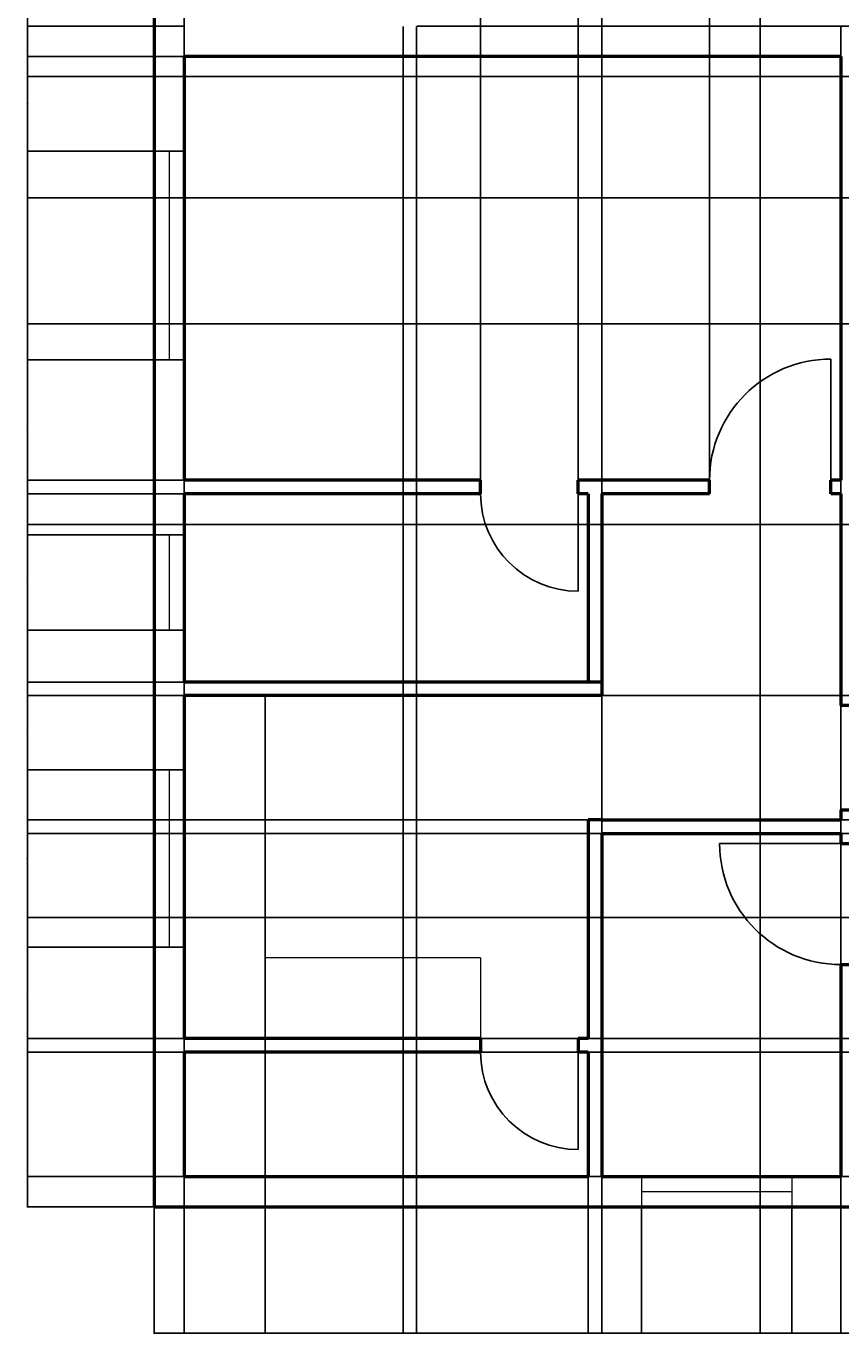
# Model space of a CAD drawing. Units: inches. Extents: x 2479 to 3284, y 2154 to 2936.
# Tile 1 of 8: x 2479 to 2721, y 2154 to 2543. Entities that reach past the tile are written whole.
import ezdxf

# ---------------------------------------------------------------- set-up
doc = ezdxf.new("R2010")
doc.units = ezdxf.units.IN
for name, color, linetype, lineweight in [('A-ANNO-DIMS', 2, 'Continuous', 18), ('A-DOOR', 3, 'Continuous', 25), ('A-FLOR-CASE', 8, 'Continuous', 18), ('A-GLAZ', 4, 'Continuous', 18), ('A-WALL', 7, 'Continuous', 50)]:
    doc.layers.add(name, color=color, linetype=linetype, lineweight=lineweight)
doc.styles.get("Standard").update_dxf_attribs({"font": 'arial.ttf'})
doc.dimstyles.get("Standard").update_dxf_attribs({"dimtxt": 0.18, "dimasz": 0.18, "dimexe": 0.18, "dimexo": 0.0625, "dimgap": 0.09, "dimtad": 0, "dimtih": 1, "dimtoh": 1, "dimdec": 4, "dimzin": 0, "dimdsep": 46, "dimtxsty": 'Standard', "dimcen": 0.09, "dimadec": 0, "dimazin": 0, "dimtfac": 1, "dimtdec": 4, "dimtofl": 0, "dimtmove": 0, "dimatfit": 3, "dimfxl": 1, "dimtolj": 1, "dimtzin": 0, "dimarcsym": 0})

# ---------------------------------------------------------------- blocks, each defined once
blk = doc.blocks.new('DOOR-SWING-29IN')
blk.add_line((29, 0), (0, 0))
blk.add_arc((29, 0), 29, 90, 180)
blk = doc.blocks.new('DOOR-SWING-36IN')
blk.add_line((36, 0), (0, 0))
blk.add_arc((36, 0), 36, 90, 180)
blk = doc.blocks.new('*D7')
at = {"layer": 'A-ANNO-DIMS', "color": 0, "lineweight": -2, "transparency": 16777216}
for p, q in [((2517.21, 2191.68), (2517.21, 2153.96)), ((3246.21, 2191.68), (3246.21, 2153.96)), ((2517.39, 2154.14), (2881.42, 2154.14)), ((3246.03, 2154.14), (2882, 2154.14))]:
    blk.add_line(p, q, dxfattribs=at)
at = {"layer": 'A-ANNO-DIMS', "color": 0, "transparency": 16777216}
for points in [[(2517.39, 2154.17), (2517.39, 2154.11), (2517.21, 2154.14)], [(3246.03, 2154.17), (3246.03, 2154.11), (3246.21, 2154.14)]]:
    blk.add_solid(points, dxfattribs=at)
at = {"layer": 'Defpoints', "color": 0, "transparency": 16777216}
for p in [(2517.21, 2191.74), (3246.21, 2191.74), (3246.21, 2154.14)]:
    blk.add_point(p, dxfattribs=at)
at = {"layer": 'A-ANNO-DIMS', "color": 0, "transparency": 16777216, "insert": (2881.71, 2154.14), "char_height": 0.18, "attachment_point": 5}
blk.add_mtext('\\A1;729', dxfattribs=at)
blk = doc.blocks.new('*D8')
at = {"layer": 'A-ANNO-DIMS', "color": 0, "lineweight": -2, "transparency": 16777216}
for p, q in [((2517.15, 2897.74), (2479.43, 2897.74)), ((2479.61, 2897.56), (2479.61, 2544.92)), ((2479.61, 2191.92), (2479.61, 2544.56)), ((2517.15, 2191.74), (2479.43, 2191.74))]:
    blk.add_line(p, q, dxfattribs=at)
at = {"layer": 'A-ANNO-DIMS', "color": 0, "transparency": 16777216}
for points in [[(2479.58, 2897.56), (2479.64, 2897.56), (2479.61, 2897.74)], [(2479.58, 2191.92), (2479.64, 2191.92), (2479.61, 2191.74)]]:
    blk.add_solid(points, dxfattribs=at)
at = {"layer": 'Defpoints', "color": 0, "transparency": 16777216}
for p in [(2479.61, 2897.74), (2517.21, 2897.74), (2517.21, 2191.74)]:
    blk.add_point(p, dxfattribs=at)
at = {"layer": 'A-ANNO-DIMS', "color": 0, "transparency": 16777216, "insert": (2479.61, 2544.74), "char_height": 0.18, "attachment_point": 5}
blk.add_mtext('\\A1;706', dxfattribs=at)
blk = doc.blocks.new('*D24')
at = {"layer": 'A-ANNO-DIMS', "color": 0, "lineweight": -2, "transparency": 16777216}
for p, q in [((2845.15, 2394.59), (2479.43, 2394.59)), ((2479.61, 2394.41), (2479.61, 2336.35)), ((2479.61, 2277.92), (2479.61, 2335.98)), ((2845.15, 2277.74), (2479.43, 2277.74))]:
    blk.add_line(p, q, dxfattribs=at)
at = {"layer": 'A-ANNO-DIMS', "color": 0, "transparency": 16777216}
for points in [[(2479.58, 2394.41), (2479.64, 2394.41), (2479.61, 2394.59)], [(2479.58, 2277.92), (2479.64, 2277.92), (2479.61, 2277.74)]]:
    blk.add_solid(points, dxfattribs=at)
at = {"layer": 'Defpoints', "color": 0, "transparency": 16777216}
for p in [(2479.61, 2394.59), (2845.21, 2394.59), (2845.21, 2277.74)]:
    blk.add_point(p, dxfattribs=at)
at = {"layer": 'A-ANNO-DIMS', "color": 0, "transparency": 16777216, "insert": (2479.61, 2336.17), "char_height": 0.18, "attachment_point": 5}
blk.add_mtext('\\A1;116.85', dxfattribs=at)
blk = doc.blocks.new('*D25')
at = {"layer": 'A-ANNO-DIMS', "color": 0, "lineweight": -2, "transparency": 16777216}
for p, q in [((2845.15, 2454.21), (2479.43, 2454.21)), ((2479.61, 2454.03), (2479.61, 2424.58)), ((2479.61, 2394.77), (2479.61, 2424.22)), ((2845.15, 2394.59), (2479.43, 2394.59))]:
    blk.add_line(p, q, dxfattribs=at)
at = {"layer": 'A-ANNO-DIMS', "color": 0, "transparency": 16777216}
for points in [[(2479.58, 2454.03), (2479.64, 2454.03), (2479.61, 2454.21)], [(2479.58, 2394.77), (2479.64, 2394.77), (2479.61, 2394.59)]]:
    blk.add_solid(points, dxfattribs=at)
at = {"layer": 'Defpoints', "color": 0, "transparency": 16777216}
for p in [(2479.61, 2454.21), (2845.21, 2454.21), (2845.21, 2394.59)]:
    blk.add_point(p, dxfattribs=at)
at = {"layer": 'A-ANNO-DIMS', "color": 0, "transparency": 16777216, "insert": (2479.61, 2424.4), "char_height": 0.18, "attachment_point": 5}
blk.add_mtext('\\A1;59.61', dxfattribs=at)
blk = doc.blocks.new('*D26')
at = {"layer": 'A-ANNO-DIMS', "color": 0, "lineweight": -2, "transparency": 16777216}
for p, q in [((2845.15, 2491.74), (2479.43, 2491.74)), ((2479.61, 2491.56), (2479.61, 2473.15)), ((2479.61, 2454.39), (2479.61, 2472.79)), ((2845.15, 2454.21), (2479.43, 2454.21))]:
    blk.add_line(p, q, dxfattribs=at)
at = {"layer": 'A-ANNO-DIMS', "color": 0, "transparency": 16777216}
for points in [[(2479.58, 2491.56), (2479.64, 2491.56), (2479.61, 2491.74)], [(2479.58, 2454.39), (2479.64, 2454.39), (2479.61, 2454.21)]]:
    blk.add_solid(points, dxfattribs=at)
at = {"layer": 'Defpoints', "color": 0, "transparency": 16777216}
for p in [(2479.61, 2491.74), (2845.21, 2491.74), (2845.21, 2454.21)]:
    blk.add_point(p, dxfattribs=at)
at = {"layer": 'A-ANNO-DIMS', "color": 0, "transparency": 16777216, "insert": (2479.61, 2472.97), "char_height": 0.18, "attachment_point": 5}
blk.add_mtext('\\A1;37.534', dxfattribs=at)
blk = doc.blocks.new('*D27')
at = {"layer": 'A-ANNO-DIMS', "color": 0, "lineweight": -2, "transparency": 16777216}
for p, q in [((2845.15, 2545.74), (2479.43, 2545.74)), ((2479.61, 2545.56), (2479.61, 2536.92)), ((2479.61, 2527.92), (2479.61, 2536.56)), ((2845.15, 2527.74), (2479.43, 2527.74))]:
    blk.add_line(p, q, dxfattribs=at)
at = {"layer": 'A-ANNO-DIMS', "color": 0, "transparency": 16777216}
for points in [[(2479.58, 2545.56), (2479.64, 2545.56), (2479.61, 2545.74)], [(2479.58, 2527.92), (2479.64, 2527.92), (2479.61, 2527.74)]]:
    blk.add_solid(points, dxfattribs=at)
at = {"layer": 'Defpoints', "color": 0, "transparency": 16777216}
for p in [(2479.61, 2545.74), (2845.21, 2545.74), (2845.21, 2527.74)]:
    blk.add_point(p, dxfattribs=at)
at = {"layer": 'A-ANNO-DIMS', "color": 0, "transparency": 16777216, "insert": (2479.61, 2536.74), "char_height": 0.18, "attachment_point": 5}
blk.add_mtext('\\A1;18', dxfattribs=at)
blk = doc.blocks.new('*D48')
at = {"layer": 'A-ANNO-DIMS', "color": 0, "lineweight": -2, "transparency": 16777216}
for p, q in [((2526.21, 2542.68), (2526.21, 2153.96)), ((2591.21, 2542.68), (2591.21, 2153.96)), ((2526.39, 2154.14), (2558.49, 2154.14)), ((2591.03, 2154.14), (2558.93, 2154.14))]:
    blk.add_line(p, q, dxfattribs=at)
at = {"layer": 'A-ANNO-DIMS', "color": 0, "transparency": 16777216}
for points in [[(2526.39, 2154.17), (2526.39, 2154.11), (2526.21, 2154.14)], [(2591.03, 2154.17), (2591.03, 2154.11), (2591.21, 2154.14)]]:
    blk.add_solid(points, dxfattribs=at)
at = {"layer": 'Defpoints', "color": 0, "transparency": 16777216}
for p in [(2526.21, 2542.74), (2591.21, 2542.74), (2591.21, 2154.14)]:
    blk.add_point(p, dxfattribs=at)
at = {"layer": 'A-ANNO-DIMS', "color": 0, "transparency": 16777216, "insert": (2558.71, 2154.14), "char_height": 0.18, "attachment_point": 5}
blk.add_mtext('\\A1;65', dxfattribs=at)
blk = doc.blocks.new('*D49')
at = {"layer": 'A-ANNO-DIMS', "color": 0, "lineweight": -2, "transparency": 16777216}
for p, q in [((2595.21, 2542.68), (2595.21, 2153.96)), ((2721.21, 2542.68), (2721.21, 2153.96)), ((2595.39, 2154.14), (2657.93, 2154.14)), ((2721.03, 2154.14), (2658.49, 2154.14))]:
    blk.add_line(p, q, dxfattribs=at)
at = {"layer": 'A-ANNO-DIMS', "color": 0, "transparency": 16777216}
for points in [[(2595.39, 2154.17), (2595.39, 2154.11), (2595.21, 2154.14)], [(2721.03, 2154.17), (2721.03, 2154.11), (2721.21, 2154.14)]]:
    blk.add_solid(points, dxfattribs=at)
at = {"layer": 'Defpoints', "color": 0, "transparency": 16777216}
for p in [(2595.21, 2542.74), (2721.21, 2542.74), (2721.21, 2154.14)]:
    blk.add_point(p, dxfattribs=at)
at = {"layer": 'A-ANNO-DIMS', "color": 0, "transparency": 16777216, "insert": (2658.21, 2154.14), "char_height": 0.18, "attachment_point": 5}
blk.add_mtext('\\A1;126', dxfattribs=at)
blk = doc.blocks.new('*D51')
at = {"layer": 'A-ANNO-DIMS', "color": 0, "lineweight": -2, "transparency": 16777216}
for p, q in [((2526.15, 2638.74), (2479.43, 2638.74)), ((2479.61, 2638.56), (2479.61, 2590.92)), ((2479.61, 2542.92), (2479.61, 2590.56)), ((2526.15, 2542.74), (2479.43, 2542.74))]:
    blk.add_line(p, q, dxfattribs=at)
at = {"layer": 'A-ANNO-DIMS', "color": 0, "transparency": 16777216}
for points in [[(2479.58, 2638.56), (2479.64, 2638.56), (2479.61, 2638.74)], [(2479.58, 2542.92), (2479.64, 2542.92), (2479.61, 2542.74)]]:
    blk.add_solid(points, dxfattribs=at)
at = {"layer": 'Defpoints', "color": 0, "transparency": 16777216}
for p in [(2479.61, 2638.74), (2526.21, 2638.74), (2526.21, 2542.74)]:
    blk.add_point(p, dxfattribs=at)
at = {"layer": 'A-ANNO-DIMS', "color": 0, "transparency": 16777216, "insert": (2479.61, 2590.74), "char_height": 0.18, "attachment_point": 5}
blk.add_mtext('\\A1;96', dxfattribs=at)
blk = doc.blocks.new('*D61')
at = {"layer": 'A-ANNO-DIMS', "color": 0, "lineweight": -2, "transparency": 16777216}
for p, q in [((2595.27, 2566.74), (3283.99, 2566.74)), ((3283.81, 2566.56), (3283.81, 2554.92)), ((3283.81, 2542.92), (3283.81, 2554.56)), ((2595.27, 2542.74), (3283.99, 2542.74))]:
    blk.add_line(p, q, dxfattribs=at)
at = {"layer": 'A-ANNO-DIMS', "color": 0, "transparency": 16777216}
for points in [[(3283.78, 2566.56), (3283.84, 2566.56), (3283.81, 2566.74)], [(3283.78, 2542.92), (3283.84, 2542.92), (3283.81, 2542.74)]]:
    blk.add_solid(points, dxfattribs=at)
at = {"layer": 'Defpoints', "color": 0, "transparency": 16777216}
for p in [(2595.21, 2566.74), (3283.81, 2566.74), (2595.21, 2542.74)]:
    blk.add_point(p, dxfattribs=at)
at = {"layer": 'A-ANNO-DIMS', "color": 0, "transparency": 16777216, "insert": (3283.81, 2554.74), "char_height": 0.18, "attachment_point": 5}
blk.add_mtext('\\A1;24', dxfattribs=at)
blk = doc.blocks.new('*D63')
at = {"layer": 'A-ANNO-DIMS', "color": 0, "lineweight": -2, "transparency": 16777216}
for p, q in [((2650.21, 2642.68), (2650.21, 2153.96)), ((2697.21, 2642.68), (2697.21, 2153.96)), ((2650.39, 2154.14), (2673.49, 2154.14)), ((2697.03, 2154.14), (2673.93, 2154.14))]:
    blk.add_line(p, q, dxfattribs=at)
at = {"layer": 'A-ANNO-DIMS', "color": 0, "transparency": 16777216}
for points in [[(2650.39, 2154.17), (2650.39, 2154.11), (2650.21, 2154.14)], [(2697.03, 2154.17), (2697.03, 2154.11), (2697.21, 2154.14)]]:
    blk.add_solid(points, dxfattribs=at)
at = {"layer": 'Defpoints', "color": 0, "transparency": 16777216}
for p in [(2650.21, 2642.74), (2697.21, 2642.74), (2697.21, 2154.14)]:
    blk.add_point(p, dxfattribs=at)
at = {"layer": 'A-ANNO-DIMS', "color": 0, "transparency": 16777216, "insert": (2673.71, 2154.14), "char_height": 0.18, "attachment_point": 5}
blk.add_mtext('\\A1;47', dxfattribs=at)
blk = doc.blocks.new('*D90')
at = {"layer": 'A-ANNO-DIMS', "color": 0, "lineweight": -2, "transparency": 16777216}
for p, q in [((2526.21, 2200.68), (2526.21, 2153.96)), ((2646.21, 2200.68), (2646.21, 2153.96)), ((2526.39, 2154.14), (2585.93, 2154.14)), ((2646.03, 2154.14), (2586.49, 2154.14))]:
    blk.add_line(p, q, dxfattribs=at)
at = {"layer": 'A-ANNO-DIMS', "color": 0, "transparency": 16777216}
for points in [[(2526.39, 2154.17), (2526.39, 2154.11), (2526.21, 2154.14)], [(2646.03, 2154.17), (2646.03, 2154.11), (2646.21, 2154.14)]]:
    blk.add_solid(points, dxfattribs=at)
at = {"layer": 'Defpoints', "color": 0, "transparency": 16777216}
for p in [(2526.21, 2200.74), (2646.21, 2200.74), (2646.21, 2154.14)]:
    blk.add_point(p, dxfattribs=at)
at = {"layer": 'A-ANNO-DIMS', "color": 0, "transparency": 16777216, "insert": (2586.21, 2154.14), "char_height": 0.18, "attachment_point": 5}
blk.add_mtext('\\A1;120', dxfattribs=at)
blk = doc.blocks.new('*D91')
at = {"layer": 'A-ANNO-DIMS', "color": 0, "lineweight": -2, "transparency": 16777216}
for p, q in [((2650.21, 2200.68), (2650.21, 2153.96)), ((2661.98, 2191.68), (2661.98, 2153.96)), ((2650.39, 2154.14), (2655.71, 2154.14)), ((2661.8, 2154.14), (2656.48, 2154.14))]:
    blk.add_line(p, q, dxfattribs=at)
at = {"layer": 'A-ANNO-DIMS', "color": 0, "transparency": 16777216}
for points in [[(2650.39, 2154.17), (2650.39, 2154.11), (2650.21, 2154.14)], [(2661.8, 2154.17), (2661.8, 2154.11), (2661.98, 2154.14)]]:
    blk.add_solid(points, dxfattribs=at)
at = {"layer": 'Defpoints', "color": 0, "transparency": 16777216}
for p in [(2650.21, 2200.74), (2661.98, 2191.74), (2661.98, 2154.14)]:
    blk.add_point(p, dxfattribs=at)
at = {"layer": 'A-ANNO-DIMS', "color": 0, "transparency": 16777216, "insert": (2656.09, 2154.14), "char_height": 0.18, "attachment_point": 5}
blk.add_mtext('\\A1;11.77', dxfattribs=at)
blk = doc.blocks.new('*D92')
at = {"layer": 'A-ANNO-DIMS', "color": 0, "lineweight": -2, "transparency": 16777216}
for p, q in [((2661.98, 2191.68), (2661.98, 2153.96)), ((2706.69, 2191.68), (2706.69, 2153.96)), ((2662.16, 2154.14), (2683.96, 2154.14)), ((2706.51, 2154.14), (2684.71, 2154.14))]:
    blk.add_line(p, q, dxfattribs=at)
at = {"layer": 'A-ANNO-DIMS', "color": 0, "transparency": 16777216}
for points in [[(2662.16, 2154.17), (2662.16, 2154.11), (2661.98, 2154.14)], [(2706.51, 2154.17), (2706.51, 2154.11), (2706.69, 2154.14)]]:
    blk.add_solid(points, dxfattribs=at)
at = {"layer": 'Defpoints', "color": 0, "transparency": 16777216}
for p in [(2661.98, 2191.74), (2706.69, 2191.74), (2706.69, 2154.14)]:
    blk.add_point(p, dxfattribs=at)
at = {"layer": 'A-ANNO-DIMS', "color": 0, "transparency": 16777216, "insert": (2684.33, 2154.14), "char_height": 0.18, "attachment_point": 5}
blk.add_mtext('\\A1;44.71', dxfattribs=at)
blk = doc.blocks.new('*D93')
at = {"layer": 'A-ANNO-DIMS', "color": 0, "lineweight": -2, "transparency": 16777216}
for p, q in [((2721.21, 2200.68), (2721.21, 2153.96)), ((2706.69, 2191.68), (2706.69, 2153.96)), ((2706.87, 2154.14), (2713.49, 2154.14)), ((2721.03, 2154.14), (2714.41, 2154.14))]:
    blk.add_line(p, q, dxfattribs=at)
at = {"layer": 'A-ANNO-DIMS', "color": 0, "transparency": 16777216}
for points in [[(2706.87, 2154.17), (2706.87, 2154.11), (2706.69, 2154.14)], [(2721.03, 2154.17), (2721.03, 2154.11), (2721.21, 2154.14)]]:
    blk.add_solid(points, dxfattribs=at)
at = {"layer": 'Defpoints', "color": 0, "transparency": 16777216}
for p in [(2721.21, 2200.74), (2706.69, 2191.74), (2721.21, 2154.14)]:
    blk.add_point(p, dxfattribs=at)
at = {"layer": 'A-ANNO-DIMS', "color": 0, "transparency": 16777216, "insert": (2713.95, 2154.14), "char_height": 0.18, "attachment_point": 5}
blk.add_mtext('\\A1;14.518', dxfattribs=at)
blk = doc.blocks.new('*D96')
at = {"layer": 'A-ANNO-DIMS', "color": 0, "lineweight": -2, "transparency": 16777216}
for p, q in [((2526.15, 2237.74), (2479.43, 2237.74)), ((2479.61, 2237.56), (2479.61, 2219.42)), ((2479.61, 2200.92), (2479.61, 2219.06)), ((2526.15, 2200.74), (2479.43, 2200.74))]:
    blk.add_line(p, q, dxfattribs=at)
at = {"layer": 'A-ANNO-DIMS', "color": 0, "transparency": 16777216}
for points in [[(2479.58, 2237.56), (2479.64, 2237.56), (2479.61, 2237.74)], [(2479.58, 2200.92), (2479.64, 2200.92), (2479.61, 2200.74)]]:
    blk.add_solid(points, dxfattribs=at)
at = {"layer": 'Defpoints', "color": 0, "transparency": 16777216}
for p in [(2479.61, 2237.74), (2526.21, 2237.74), (2526.21, 2200.74)]:
    blk.add_point(p, dxfattribs=at)
at = {"layer": 'A-ANNO-DIMS', "color": 0, "transparency": 16777216, "insert": (2479.61, 2219.24), "char_height": 0.18, "attachment_point": 5}
blk.add_mtext('\\A1;37', dxfattribs=at)
blk = doc.blocks.new('*D97')
at = {"layer": 'A-ANNO-DIMS', "color": 0, "lineweight": -2, "transparency": 16777216}
for p, q in [((2526.15, 2268.88), (2479.43, 2268.88)), ((2479.61, 2268.7), (2479.61, 2255.49)), ((2479.61, 2241.92), (2479.61, 2255.13)), ((2526.15, 2241.74), (2479.43, 2241.74))]:
    blk.add_line(p, q, dxfattribs=at)
at = {"layer": 'A-ANNO-DIMS', "color": 0, "transparency": 16777216}
for points in [[(2479.58, 2268.7), (2479.64, 2268.7), (2479.61, 2268.88)], [(2479.58, 2241.92), (2479.64, 2241.92), (2479.61, 2241.74)]]:
    blk.add_solid(points, dxfattribs=at)
at = {"layer": 'Defpoints', "color": 0, "transparency": 16777216}
for p in [(2479.61, 2268.88), (2526.21, 2268.88), (2526.21, 2241.74)]:
    blk.add_point(p, dxfattribs=at)
at = {"layer": 'A-ANNO-DIMS', "color": 0, "transparency": 16777216, "insert": (2479.61, 2255.31), "char_height": 0.18, "attachment_point": 5}
blk.add_mtext('\\A1;27.14', dxfattribs=at)
blk = doc.blocks.new('*D98')
at = {"layer": 'A-ANNO-DIMS', "color": 0, "lineweight": -2, "transparency": 16777216}
for p, q in [((2526.15, 2321.65), (2479.43, 2321.65)), ((2479.61, 2321.47), (2479.61, 2295.44)), ((2479.61, 2269.06), (2479.61, 2295.08)), ((2526.15, 2268.88), (2479.43, 2268.88))]:
    blk.add_line(p, q, dxfattribs=at)
at = {"layer": 'A-ANNO-DIMS', "color": 0, "transparency": 16777216}
for points in [[(2479.58, 2321.47), (2479.64, 2321.47), (2479.61, 2321.65)], [(2479.58, 2269.06), (2479.64, 2269.06), (2479.61, 2268.88)]]:
    blk.add_solid(points, dxfattribs=at)
at = {"layer": 'Defpoints', "color": 0, "transparency": 16777216}
for p in [(2479.61, 2321.65), (2526.21, 2321.65), (2526.21, 2268.88)]:
    blk.add_point(p, dxfattribs=at)
at = {"layer": 'A-ANNO-DIMS', "color": 0, "transparency": 16777216, "insert": (2479.61, 2295.26), "char_height": 0.18, "attachment_point": 5}
blk.add_mtext('\\A1;52.76', dxfattribs=at)
blk = doc.blocks.new('*D99')
at = {"layer": 'A-ANNO-DIMS', "color": 0, "lineweight": -2, "transparency": 16777216}
for p, q in [((2526.15, 2343.74), (2479.43, 2343.74)), ((2479.61, 2343.56), (2479.61, 2332.87)), ((2479.61, 2321.83), (2479.61, 2332.51)), ((2526.15, 2321.65), (2479.43, 2321.65))]:
    blk.add_line(p, q, dxfattribs=at)
at = {"layer": 'A-ANNO-DIMS', "color": 0, "transparency": 16777216}
for points in [[(2479.58, 2343.56), (2479.64, 2343.56), (2479.61, 2343.74)], [(2479.58, 2321.83), (2479.64, 2321.83), (2479.61, 2321.65)]]:
    blk.add_solid(points, dxfattribs=at)
at = {"layer": 'Defpoints', "color": 0, "transparency": 16777216}
for p in [(2479.61, 2343.74), (2526.21, 2343.74), (2526.21, 2321.65)]:
    blk.add_point(p, dxfattribs=at)
at = {"layer": 'A-ANNO-DIMS', "color": 0, "transparency": 16777216, "insert": (2479.61, 2332.69), "char_height": 0.18, "attachment_point": 5}
blk.add_mtext('\\A1;22.095', dxfattribs=at)
blk = doc.blocks.new('*D100')
at = {"layer": 'A-ANNO-DIMS', "color": 0, "lineweight": -2, "transparency": 16777216}
for p, q in [((2526.15, 2363.18), (2479.43, 2363.18)), ((2479.61, 2363), (2479.61, 2355.64)), ((2479.61, 2347.92), (2479.61, 2355.28)), ((2526.15, 2347.74), (2479.43, 2347.74))]:
    blk.add_line(p, q, dxfattribs=at)
at = {"layer": 'A-ANNO-DIMS', "color": 0, "transparency": 16777216}
for points in [[(2479.58, 2363), (2479.64, 2363), (2479.61, 2363.18)], [(2479.58, 2347.92), (2479.64, 2347.92), (2479.61, 2347.74)]]:
    blk.add_solid(points, dxfattribs=at)
at = {"layer": 'Defpoints', "color": 0, "transparency": 16777216}
for p in [(2479.61, 2363.18), (2526.21, 2363.18), (2526.21, 2347.74)]:
    blk.add_point(p, dxfattribs=at)
at = {"layer": 'A-ANNO-DIMS', "color": 0, "transparency": 16777216, "insert": (2479.61, 2355.46), "char_height": 0.18, "attachment_point": 5}
blk.add_mtext('\\A1;15.44', dxfattribs=at)
blk = doc.blocks.new('*D101')
at = {"layer": 'A-ANNO-DIMS', "color": 0, "lineweight": -2, "transparency": 16777216}
for p, q in [((2526.15, 2391.55), (2479.43, 2391.55)), ((2479.61, 2391.37), (2479.61, 2377.55)), ((2479.61, 2363.36), (2479.61, 2377.18)), ((2526.15, 2363.18), (2479.43, 2363.18))]:
    blk.add_line(p, q, dxfattribs=at)
at = {"layer": 'A-ANNO-DIMS', "color": 0, "transparency": 16777216}
for points in [[(2479.58, 2391.37), (2479.64, 2391.37), (2479.61, 2391.55)], [(2479.58, 2363.36), (2479.64, 2363.36), (2479.61, 2363.18)]]:
    blk.add_solid(points, dxfattribs=at)
at = {"layer": 'Defpoints', "color": 0, "transparency": 16777216}
for p in [(2479.61, 2391.55), (2526.21, 2391.55), (2526.21, 2363.18)]:
    blk.add_point(p, dxfattribs=at)
at = {"layer": 'A-ANNO-DIMS', "color": 0, "transparency": 16777216, "insert": (2479.61, 2377.37), "char_height": 0.18, "attachment_point": 5}
blk.add_mtext('\\A1;28.376', dxfattribs=at)
blk = doc.blocks.new('*D102')
at = {"layer": 'A-ANNO-DIMS', "color": 0, "lineweight": -2, "transparency": 16777216}
for p, q in [((2526.15, 2403.74), (2479.43, 2403.74)), ((2479.61, 2403.56), (2479.61, 2397.83)), ((2479.61, 2391.73), (2479.61, 2397.47)), ((2526.15, 2391.55), (2479.43, 2391.55))]:
    blk.add_line(p, q, dxfattribs=at)
at = {"layer": 'A-ANNO-DIMS', "color": 0, "transparency": 16777216}
for points in [[(2479.58, 2403.56), (2479.64, 2403.56), (2479.61, 2403.74)], [(2479.58, 2391.73), (2479.64, 2391.73), (2479.61, 2391.55)]]:
    blk.add_solid(points, dxfattribs=at)
at = {"layer": 'Defpoints', "color": 0, "transparency": 16777216}
for p in [(2479.61, 2403.74), (2526.21, 2403.74), (2526.21, 2391.55)]:
    blk.add_point(p, dxfattribs=at)
at = {"layer": 'A-ANNO-DIMS', "color": 0, "transparency": 16777216, "insert": (2479.61, 2397.65), "char_height": 0.18, "attachment_point": 5}
blk.add_mtext('\\A1;12.185', dxfattribs=at)
blk = doc.blocks.new('*D103')
at = {"layer": 'A-ANNO-DIMS', "color": 0, "lineweight": -2, "transparency": 16777216}
for p, q in [((2526.15, 2443.49), (2479.43, 2443.49)), ((2479.61, 2443.31), (2479.61, 2425.8)), ((2479.61, 2407.92), (2479.61, 2425.43)), ((2526.15, 2407.74), (2479.43, 2407.74))]:
    blk.add_line(p, q, dxfattribs=at)
at = {"layer": 'A-ANNO-DIMS', "color": 0, "transparency": 16777216}
for points in [[(2479.58, 2443.31), (2479.64, 2443.31), (2479.61, 2443.49)], [(2479.58, 2407.92), (2479.64, 2407.92), (2479.61, 2407.74)]]:
    blk.add_solid(points, dxfattribs=at)
at = {"layer": 'Defpoints', "color": 0, "transparency": 16777216}
for p in [(2479.61, 2443.49), (2526.21, 2443.49), (2526.21, 2407.74)]:
    blk.add_point(p, dxfattribs=at)
at = {"layer": 'A-ANNO-DIMS', "color": 0, "transparency": 16777216, "insert": (2479.61, 2425.61), "char_height": 0.18, "attachment_point": 5}
blk.add_mtext('\\A1;35.75', dxfattribs=at)
blk = doc.blocks.new('*D104')
at = {"layer": 'A-ANNO-DIMS', "color": 0, "lineweight": -2, "transparency": 16777216}
for p, q in [((2526.15, 2505.53), (2479.43, 2505.53)), ((2479.61, 2505.35), (2479.61, 2474.69)), ((2479.61, 2443.67), (2479.61, 2474.33)), ((2526.15, 2443.49), (2479.43, 2443.49))]:
    blk.add_line(p, q, dxfattribs=at)
at = {"layer": 'A-ANNO-DIMS', "color": 0, "transparency": 16777216}
for points in [[(2479.58, 2505.35), (2479.64, 2505.35), (2479.61, 2505.53)], [(2479.58, 2443.67), (2479.64, 2443.67), (2479.61, 2443.49)]]:
    blk.add_solid(points, dxfattribs=at)
at = {"layer": 'Defpoints', "color": 0, "transparency": 16777216}
for p in [(2479.61, 2505.53), (2526.21, 2505.53), (2526.21, 2443.49)]:
    blk.add_point(p, dxfattribs=at)
at = {"layer": 'A-ANNO-DIMS', "color": 0, "transparency": 16777216, "insert": (2479.61, 2474.51), "char_height": 0.18, "attachment_point": 5}
blk.add_mtext('\\A1;62.05', dxfattribs=at)
blk = doc.blocks.new('*D105')
at = {"layer": 'A-ANNO-DIMS', "color": 0, "lineweight": -2, "transparency": 16777216}
for p, q in [((2526.15, 2533.74), (2479.43, 2533.74)), ((2479.61, 2533.56), (2479.61, 2519.82)), ((2479.61, 2505.71), (2479.61, 2519.46)), ((2526.15, 2505.53), (2479.43, 2505.53))]:
    blk.add_line(p, q, dxfattribs=at)
at = {"layer": 'A-ANNO-DIMS', "color": 0, "transparency": 16777216}
for points in [[(2479.58, 2533.56), (2479.64, 2533.56), (2479.61, 2533.74)], [(2479.58, 2505.71), (2479.64, 2505.71), (2479.61, 2505.53)]]:
    blk.add_solid(points, dxfattribs=at)
at = {"layer": 'Defpoints', "color": 0, "transparency": 16777216}
for p in [(2479.61, 2533.74), (2526.21, 2533.74), (2526.21, 2505.53)]:
    blk.add_point(p, dxfattribs=at)
at = {"layer": 'A-ANNO-DIMS', "color": 0, "transparency": 16777216, "insert": (2479.61, 2519.64), "char_height": 0.18, "attachment_point": 5}
blk.add_mtext('\\A1;28.205', dxfattribs=at)
blk = doc.blocks.new('*D109')
at = {"layer": 'A-ANNO-DIMS', "color": 0, "lineweight": -2, "transparency": 16777216}
for p, q in [((2526.21, 2407.8), (2526.21, 2935.52)), ((2526.39, 2935.34), (2569.99, 2935.34)), ((2614.03, 2935.34), (2570.43, 2935.34)), ((2614.21, 2407.8), (2614.21, 2935.52))]:
    blk.add_line(p, q, dxfattribs=at)
at = {"layer": 'A-ANNO-DIMS', "color": 0, "transparency": 16777216}
for points in [[(2526.39, 2935.37), (2526.39, 2935.31), (2526.21, 2935.34)], [(2614.03, 2935.37), (2614.03, 2935.31), (2614.21, 2935.34)]]:
    blk.add_solid(points, dxfattribs=at)
at = {"layer": 'Defpoints', "color": 0, "transparency": 16777216}
for p in [(2614.21, 2935.34), (2526.21, 2407.74), (2614.21, 2407.74)]:
    blk.add_point(p, dxfattribs=at)
at = {"layer": 'A-ANNO-DIMS', "color": 0, "transparency": 16777216, "insert": (2570.21, 2935.34), "char_height": 0.18, "attachment_point": 5}
blk.add_mtext('\\A1;88', dxfattribs=at)
blk = doc.blocks.new('*D110')
at = {"layer": 'A-ANNO-DIMS', "color": 0, "lineweight": -2, "transparency": 16777216}
for p, q in [((2643.21, 2407.8), (2643.21, 2935.52)), ((2643.39, 2935.34), (2662.49, 2935.34)), ((2682.03, 2935.34), (2662.93, 2935.34)), ((2682.21, 2407.8), (2682.21, 2935.52))]:
    blk.add_line(p, q, dxfattribs=at)
at = {"layer": 'A-ANNO-DIMS', "color": 0, "transparency": 16777216}
for points in [[(2643.39, 2935.37), (2643.39, 2935.31), (2643.21, 2935.34)], [(2682.03, 2935.37), (2682.03, 2935.31), (2682.21, 2935.34)]]:
    blk.add_solid(points, dxfattribs=at)
at = {"layer": 'Defpoints', "color": 0, "transparency": 16777216}
for p in [(2682.21, 2935.34), (2643.21, 2407.74), (2682.21, 2407.74)]:
    blk.add_point(p, dxfattribs=at)
at = {"layer": 'A-ANNO-DIMS', "color": 0, "transparency": 16777216, "insert": (2662.71, 2935.34), "char_height": 0.18, "attachment_point": 5}
blk.add_mtext('\\A1;39', dxfattribs=at)
blk = doc.blocks.new('*D111')
at = {"layer": 'A-ANNO-DIMS', "color": 0, "lineweight": -2, "transparency": 16777216}
for p, q in [((2526.21, 2343.68), (2526.21, 2153.96)), ((2550.21, 2343.68), (2550.21, 2153.96)), ((2526.39, 2154.14), (2537.99, 2154.14)), ((2550.03, 2154.14), (2538.43, 2154.14))]:
    blk.add_line(p, q, dxfattribs=at)
at = {"layer": 'A-ANNO-DIMS', "color": 0, "transparency": 16777216}
for points in [[(2526.39, 2154.17), (2526.39, 2154.11), (2526.21, 2154.14)], [(2550.03, 2154.17), (2550.03, 2154.11), (2550.21, 2154.14)]]:
    blk.add_solid(points, dxfattribs=at)
at = {"layer": 'Defpoints', "color": 0, "transparency": 16777216}
for p in [(2526.21, 2343.74), (2550.21, 2343.74), (2550.21, 2154.14)]:
    blk.add_point(p, dxfattribs=at)
at = {"layer": 'A-ANNO-DIMS', "color": 0, "transparency": 16777216, "insert": (2538.21, 2154.14), "char_height": 0.18, "attachment_point": 5}
blk.add_mtext('\\A1;24', dxfattribs=at)
blk = doc.blocks.new('*D128')
at = {"layer": 'A-ANNO-DIMS', "color": 0, "lineweight": -2, "transparency": 16777216}
for p, q in [((3032.15, 2237.74), (2479.43, 2237.74)), ((2479.61, 2237.56), (2479.61, 2219.42)), ((2479.61, 2200.92), (2479.61, 2219.06)), ((3032.15, 2200.74), (2479.43, 2200.74))]:
    blk.add_line(p, q, dxfattribs=at)
at = {"layer": 'A-ANNO-DIMS', "color": 0, "transparency": 16777216}
for points in [[(2479.58, 2237.56), (2479.64, 2237.56), (2479.61, 2237.74)], [(2479.58, 2200.92), (2479.64, 2200.92), (2479.61, 2200.74)]]:
    blk.add_solid(points, dxfattribs=at)
at = {"layer": 'Defpoints', "color": 0, "transparency": 16777216}
for p in [(2479.61, 2237.74), (3032.21, 2237.74), (3032.21, 2200.74)]:
    blk.add_point(p, dxfattribs=at)
at = {"layer": 'A-ANNO-DIMS', "color": 0, "transparency": 16777216, "insert": (2479.61, 2219.24), "char_height": 0.18, "attachment_point": 5}
blk.add_mtext('\\A1;37', dxfattribs=at)
blk = doc.blocks.new('*D129')
at = {"layer": 'A-ANNO-DIMS', "color": 0, "lineweight": -2, "transparency": 16777216}
for p, q in [((3041.15, 2302.74), (2479.43, 2302.74)), ((2479.61, 2302.56), (2479.61, 2272.42)), ((2479.61, 2241.92), (2479.61, 2272.06)), ((2911.15, 2241.74), (2479.43, 2241.74))]:
    blk.add_line(p, q, dxfattribs=at)
at = {"layer": 'A-ANNO-DIMS', "color": 0, "transparency": 16777216}
for points in [[(2479.58, 2302.56), (2479.64, 2302.56), (2479.61, 2302.74)], [(2479.58, 2241.92), (2479.64, 2241.92), (2479.61, 2241.74)]]:
    blk.add_solid(points, dxfattribs=at)
at = {"layer": 'Defpoints', "color": 0, "transparency": 16777216}
for p in [(2479.61, 2302.74), (3041.21, 2302.74), (2911.21, 2241.74)]:
    blk.add_point(p, dxfattribs=at)
at = {"layer": 'A-ANNO-DIMS', "color": 0, "transparency": 16777216, "insert": (2479.61, 2272.24), "char_height": 0.18, "attachment_point": 5}
blk.add_mtext('\\A1;61', dxfattribs=at)
blk = doc.blocks.new('*D130')
at = {"layer": 'A-ANNO-DIMS', "color": 0, "lineweight": -2, "transparency": 16777216}
for p, q in [((2911.15, 2343.74), (2479.43, 2343.74)), ((2479.61, 2343.56), (2479.61, 2325.42)), ((2479.61, 2306.92), (2479.61, 2325.06)), ((3041.15, 2306.74), (2479.43, 2306.74))]:
    blk.add_line(p, q, dxfattribs=at)
at = {"layer": 'A-ANNO-DIMS', "color": 0, "transparency": 16777216}
for points in [[(2479.58, 2343.56), (2479.64, 2343.56), (2479.61, 2343.74)], [(2479.58, 2306.92), (2479.64, 2306.92), (2479.61, 2306.74)]]:
    blk.add_solid(points, dxfattribs=at)
at = {"layer": 'Defpoints', "color": 0, "transparency": 16777216}
for p in [(2479.61, 2343.74), (2911.21, 2343.74), (3041.21, 2306.74)]:
    blk.add_point(p, dxfattribs=at)
at = {"layer": 'A-ANNO-DIMS', "color": 0, "transparency": 16777216, "insert": (2479.61, 2325.24), "char_height": 0.18, "attachment_point": 5}
blk.add_mtext('\\A1;37', dxfattribs=at)

msp = doc.modelspace()

# ---------------------------------------------------------------- linework, layer by layer
at = {"layer": 'A-FLOR-CASE'}
for p, q in [((2550.2088, 2343.7397), (2550.2088, 2265.7397)), ((2614.2088, 2265.7397), (2550.2088, 2265.7397)), ((2614.2088, 2265.7397), (2614.2088, 2241.7397))]:
    msp.add_line(p, q, dxfattribs=at)
at = {"layer": 'A-GLAZ'}
for p, q in [((2526.2088, 2505.5344), (2517.2088, 2505.5344)), ((2521.7088, 2505.5344), (2521.7088, 2443.4885)), ((2526.2088, 2443.4885), (2517.2088, 2443.4885)), ((2526.2088, 2391.5546), (2517.2088, 2391.5546)), ((2521.7088, 2391.5546), (2521.7088, 2363.1784)), ((2526.2088, 2363.1784), (2517.2088, 2363.1784)), ((2526.2088, 2321.6451), (2517.2088, 2321.6451)), ((2521.7088, 2321.6451), (2521.7088, 2268.8805)), ((2526.2088, 2268.8805), (2517.2088, 2268.8805)), ((2661.9792, 2200.7397), (2661.9792, 2191.7397)), ((2706.6907, 2200.7397), (2706.6907, 2191.7397)), ((2661.9792, 2196.2397), (2706.6907, 2196.2397))]:
    msp.add_line(p, q, dxfattribs=at)
at = {"layer": 'A-WALL'}
for p, q in [((2517.2088, 2897.7397), (2517.2088, 2191.7397)), ((2526.2088, 2533.7397), (2526.2088, 2407.7397)), ((2721.2088, 2533.7397), (2526.2088, 2533.7397)), ((2721.2088, 2533.7397), (2721.2088, 2407.7397)), ((2614.2088, 2407.7397), (2526.2088, 2407.7397)), ((2614.2088, 2403.7397), (2614.2088, 2407.7397)), ((2682.2088, 2407.7397), (2643.2088, 2407.7397)), ((2643.2088, 2403.7397), (2643.2088, 2407.7397)), ((2682.2088, 2403.7397), (2682.2088, 2407.7397)), ((2721.2088, 2407.7397), (2718.2088, 2407.7397)), ((2718.2088, 2403.7397), (2718.2088, 2407.7397)), ((2526.2088, 2403.7397), (2526.2088, 2347.7397)), ((2614.2088, 2403.7397), (2526.2088, 2403.7397)), ((2646.2088, 2403.7397), (2643.2088, 2403.7397)), ((2646.2088, 2403.7397), (2646.2088, 2347.7397)), ((2650.2088, 2403.7397), (2650.2088, 2347.7397)), ((2682.2088, 2403.7397), (2650.2088, 2403.7397)), ((2721.2088, 2403.7397), (2718.2088, 2403.7397)), ((2721.2088, 2403.7397), (2721.2088, 2340.7397)), ((2650.2088, 2347.7397), (2526.2088, 2347.7397)), ((2650.2088, 2347.7397), (2650.2088, 2343.7397)), ((2650.2088, 2343.7397), (2526.2088, 2343.7397)), ((2526.2088, 2343.7397), (2526.2088, 2241.7397)), ((2727.2088, 2340.7397), (2721.2088, 2340.7397)), ((2721.2088, 2309.7397), (2727.2088, 2309.7397)), ((2721.2088, 2309.7397), (2721.2088, 2306.7397)), ((2646.2088, 2306.7397), (2646.2088, 2241.7397)), ((2650.2088, 2306.7397), (2646.2088, 2306.7397)), ((2650.2088, 2306.7397), (2721.2088, 2306.7397)), ((2650.2088, 2302.7397), (2721.2088, 2302.7397)), ((2650.2088, 2302.7397), (2650.2088, 2200.7397)), ((2721.2088, 2302.7397), (2721.2088, 2299.7397)), ((2721.2088, 2299.7397), (2727.2088, 2299.7397)), ((2721.2088, 2263.7397), (2727.2088, 2263.7397)), ((2721.2088, 2263.7397), (2721.2088, 2200.7397)), ((2614.2088, 2241.7397), (2526.2088, 2241.7397)), ((2614.2088, 2241.7397), (2614.2088, 2237.7397)), ((2646.2088, 2241.7397), (2643.2088, 2241.7397)), ((2643.2088, 2241.7397), (2643.2088, 2237.7397)), ((2526.2088, 2237.7397), (2526.2088, 2200.7397)), ((2614.2088, 2237.7397), (2526.2088, 2237.7397)), ((2646.2088, 2237.7397), (2643.2088, 2237.7397)), ((2646.2088, 2237.7397), (2646.2088, 2200.7397)), ((2526.2088, 2200.7397), (2646.2088, 2200.7397)), ((2650.2088, 2200.7397), (2721.2088, 2200.7397)), ((2517.2088, 2191.7397), (3246.2088, 2191.7397))]:
    msp.add_line(p, q, dxfattribs=at)

# ---------------------------------------------------------------- block references
at = {"layer": 'A-DOOR', "extrusion": (0, 0, -1), "zscale": -1}
for p, rotation in [((-2718.2088, 2443.7397), 269.9999999999993), ((-2685.2088, 2299.7397), 180)]:
    msp.add_blockref('DOOR-SWING-36IN', p, dxfattribs=dict(at, rotation=rotation))
at = {"layer": 'A-DOOR'}
for p, rotation in [((2643.2088, 2374.7397), 90.00000000000179), ((2643.2088, 2208.7397), 90.00000000000225)]:
    msp.add_blockref('DOOR-SWING-29IN', p, dxfattribs=dict(at, rotation=rotation))

# ---------------------------------------------------------------- dimensions: what is measured, and where the dimension line sits
at = {"layer": 'A-ANNO-DIMS'}
for base, p1, p2, override, picture, middle in [((2614.2088, 2935.3397), (2526.2088, 2407.7397), (2614.2088, 2407.7397), {"dimdec": 0, "dimlfac": 1, "dimrnd": 0, "dimzin": 0, "dimdsep": 46, "dimlunit": 2}, '*D109', (2570.2088, 2935.3397)), ((2682.2088, 2935.3397), (2643.2088, 2407.7397), (2682.2088, 2407.7397), {"dimdec": 0, "dimlfac": 1, "dimrnd": 0, "dimzin": 0, "dimdsep": 46, "dimlunit": 2}, '*D110', (2662.7088, 2935.3397)), ((2697.2088, 2154.1397), (2650.2088, 2642.7397), (2697.2088, 2642.7397), {"dimdec": 0, "dimlfac": 1, "dimrnd": 0, "dimzin": 0, "dimdsep": 46, "dimlunit": 2}, '*D63', (2673.7088, 2154.1397)), ((2591.2088, 2154.1397), (2526.2088, 2542.7397), (2591.2088, 2542.7397), {"dimdec": 0, "dimlfac": 1, "dimrnd": 0, "dimzin": 0, "dimdsep": 46, "dimlunit": 2}, '*D48', (2558.7088, 2154.1397)), ((2721.2088, 2154.1397), (2595.2088, 2542.7397), (2721.2088, 2542.7397), {"dimdec": 0, "dimlfac": 1, "dimrnd": 0, "dimzin": 0, "dimdsep": 46, "dimlunit": 2}, '*D49', (2658.2088, 2154.1397)), ((2550.2088, 2154.1397), (2526.2088, 2343.7397), (2550.2088, 2343.7397), {"dimdec": 0, "dimlfac": 1, "dimrnd": 0, "dimzin": 0, "dimdsep": 46, "dimlunit": 2}, '*D111', (2538.2088, 2154.1397)), ((2646.2088, 2154.1397), (2526.2088, 2200.7397), (2646.2088, 2200.7397), {"dimdec": 0, "dimlfac": 1, "dimrnd": 0, "dimzin": 0, "dimdsep": 46, "dimlunit": 2}, '*D90', (2586.2088, 2154.1397)), ((2661.9792, 2154.1397), (2650.2088, 2200.7397), (2661.9792, 2191.7397), {"dimdec": 2, "dimlfac": 1, "dimrnd": 0, "dimzin": 0, "dimdsep": 46, "dimlunit": 2}, '*D91', (2656.094, 2154.1397)), ((2721.2088, 2154.1397), (2706.6907, 2191.7397), (2721.2088, 2200.7397), {"dimdec": 3, "dimlfac": 1, "dimrnd": 0, "dimzin": 0, "dimdsep": 46, "dimlunit": 2}, '*D93', (2713.9498, 2154.1397)), ((3246.2088, 2154.1397), (2517.2088, 2191.7397), (3246.2088, 2191.7397), {"dimdec": 0, "dimlfac": 1, "dimrnd": 0, "dimzin": 0, "dimdsep": 46, "dimlunit": 2}, '*D7', (2881.7088, 2154.1397)), ((2706.6907, 2154.1397), (2661.9792, 2191.7397), (2706.6907, 2191.7397), {"dimdec": 2, "dimlfac": 1, "dimrnd": 0, "dimzin": 0, "dimdsep": 46, "dimlunit": 2}, '*D92', (2684.335, 2154.1397))]:
    dim = msp.add_linear_dim(base=base, p1=p1, p2=p2, dimstyle='Standard', override=override, dxfattribs=at)
    dim.commit()
    dim.dimension.update_dxf_attribs({"geometry": picture, "text_midpoint": middle})
for base, p1, p2, override, picture, middle in [((2479.6088, 2897.7397), (2517.2088, 2191.7397), (2517.2088, 2897.7397), {"dimdec": 0, "dimlfac": 1, "dimrnd": 0, "dimzin": 0, "dimdsep": 46, "dimlunit": 2}, '*D8', (2479.6088, 2544.7397)), ((2479.6088, 2638.7397), (2526.2088, 2542.7397), (2526.2088, 2638.7397), {"dimdec": 0, "dimlfac": 1, "dimrnd": 0, "dimzin": 0, "dimdsep": 46, "dimlunit": 2}, '*D51', (2479.6088, 2590.7397)), ((3283.8088, 2566.7397), (2595.2088, 2542.7397), (2595.2088, 2566.7397), {"dimdec": 0, "dimlfac": 1, "dimrnd": 0, "dimzin": 0, "dimdsep": 46, "dimlunit": 2}, '*D61', (3283.8088, 2554.7397)), ((2479.6088, 2545.7397), (2845.2088, 2527.7397), (2845.2088, 2545.7397), {"dimdec": 0, "dimlfac": 1, "dimrnd": 0, "dimzin": 0, "dimdsep": 46, "dimlunit": 2}, '*D27', (2479.6088, 2536.7397)), ((2479.6088, 2533.7397), (2526.2088, 2505.5344), (2526.2088, 2533.7397), {"dimdec": 3, "dimlfac": 1, "dimrnd": 0, "dimzin": 0, "dimdsep": 46, "dimlunit": 2}, '*D105', (2479.6088, 2519.6371)), ((2479.6088, 2505.5344), (2526.2088, 2443.4885), (2526.2088, 2505.5344), {"dimdec": 2, "dimlfac": 1, "dimrnd": 0, "dimzin": 0, "dimdsep": 46, "dimlunit": 2}, '*D104', (2479.6088, 2474.5114)), ((2479.6088, 2491.7397), (2845.2088, 2454.2054), (2845.2088, 2491.7397), {"dimdec": 3, "dimlfac": 1, "dimrnd": 0, "dimzin": 0, "dimdsep": 46, "dimlunit": 2}, '*D26', (2479.6088, 2472.9726)), ((2479.6088, 2454.2054), (2845.2088, 2394.5937), (2845.2088, 2454.2054), {"dimdec": 2, "dimlfac": 1, "dimrnd": 0, "dimzin": 0, "dimdsep": 46, "dimlunit": 2}, '*D25', (2479.6088, 2424.3996)), ((2479.6088, 2443.4885), (2526.2088, 2407.7397), (2526.2088, 2443.4885), {"dimdec": 2, "dimlfac": 1, "dimrnd": 0, "dimzin": 0, "dimdsep": 46, "dimlunit": 2}, '*D103', (2479.6088, 2425.6141)), ((2479.6088, 2403.7397), (2526.2088, 2391.5546), (2526.2088, 2403.7397), {"dimdec": 3, "dimlfac": 1, "dimrnd": 0, "dimzin": 0, "dimdsep": 46, "dimlunit": 2}, '*D102', (2479.6088, 2397.6472)), ((2479.6088, 2394.5937), (2845.2088, 2277.7397), (2845.2088, 2394.5937), {"dimdec": 2, "dimlfac": 1, "dimrnd": 0, "dimzin": 0, "dimdsep": 46, "dimlunit": 2}, '*D24', (2479.6088, 2336.1667)), ((2479.6088, 2391.5546), (2526.2088, 2363.1784), (2526.2088, 2391.5546), {"dimdec": 3, "dimlfac": 1, "dimrnd": 0, "dimzin": 0, "dimdsep": 46, "dimlunit": 2}, '*D101', (2479.6088, 2377.3665)), ((2479.6088, 2363.1784), (2526.2088, 2347.7397), (2526.2088, 2363.1784), {"dimdec": 2, "dimlfac": 1, "dimrnd": 0, "dimzin": 0, "dimdsep": 46, "dimlunit": 2}, '*D100', (2479.6088, 2355.4591)), ((2479.6088, 2343.7397), (2526.2088, 2321.6451), (2526.2088, 2343.7397), {"dimdec": 3, "dimlfac": 1, "dimrnd": 0, "dimzin": 0, "dimdsep": 46, "dimlunit": 2}, '*D99', (2479.6088, 2332.6924)), ((2479.6088, 2343.7397), (3041.2088, 2306.7397), (2911.2088, 2343.7397), {"dimdec": 0, "dimlfac": 1, "dimrnd": 0, "dimzin": 0, "dimdsep": 46, "dimlunit": 2}, '*D130', (2479.6088, 2325.2397)), ((2479.6088, 2321.6451), (2526.2088, 2268.8805), (2526.2088, 2321.6451), {"dimdec": 2, "dimlfac": 1, "dimrnd": 0, "dimzin": 0, "dimdsep": 46, "dimlunit": 2}, '*D98', (2479.6088, 2295.2628)), ((2479.6088, 2302.7397), (2911.2088, 2241.7397), (3041.2088, 2302.7397), {"dimdec": 0, "dimlfac": 1, "dimrnd": 0, "dimzin": 0, "dimdsep": 46, "dimlunit": 2}, '*D129', (2479.6088, 2272.2397)), ((2479.6088, 2268.8805), (2526.2088, 2241.7397), (2526.2088, 2268.8805), {"dimdec": 2, "dimlfac": 1, "dimrnd": 0, "dimzin": 0, "dimdsep": 46, "dimlunit": 2}, '*D97', (2479.6088, 2255.3101)), ((2479.6088, 2237.7397), (2526.2088, 2200.7397), (2526.2088, 2237.7397), {"dimdec": 0, "dimlfac": 1, "dimrnd": 0, "dimzin": 0, "dimdsep": 46, "dimlunit": 2}, '*D96', (2479.6088, 2219.2397)), ((2479.6088, 2237.7397), (3032.2088, 2200.7397), (3032.2088, 2237.7397), {"dimdec": 0, "dimlfac": 1, "dimrnd": 0, "dimzin": 0, "dimdsep": 46, "dimlunit": 2}, '*D128', (2479.6088, 2219.2397))]:
    dim = msp.add_linear_dim(base=base, p1=p1, p2=p2, angle=90, dimstyle='Standard', override=override, dxfattribs=at)
    dim.commit()
    dim.dimension.update_dxf_attribs({"geometry": picture, "text_midpoint": middle})

doc.saveas('drawing.dxf')
